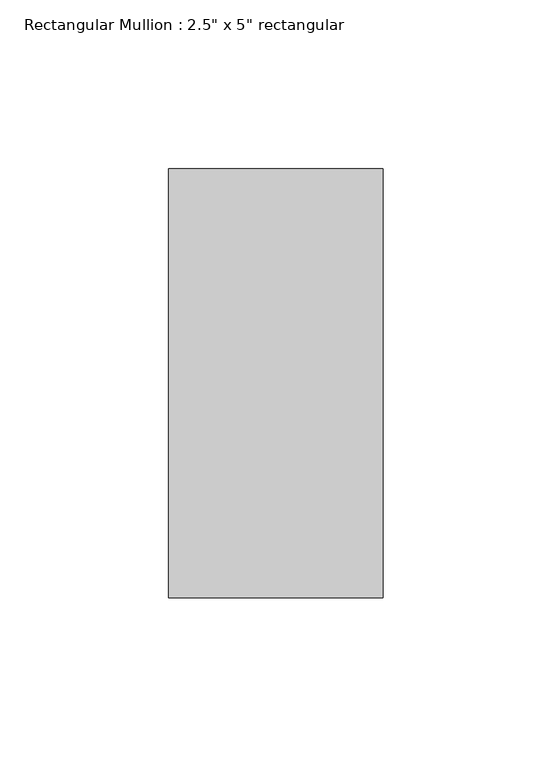
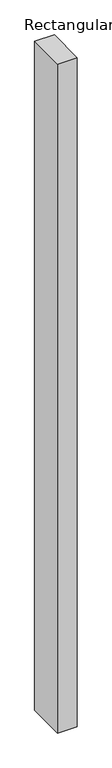
"""IFC4 building model written with IfcOpenShell, lengths in millimetres: member geometry."""

from ifc_helpers import new_model, si_unit, frame, origin, place, context, project, spatial, polyline, outline, extrude, source, transform, mapped, element, save


def member_cc169a76(model_context):
    return source(origin(), model_context, "Body", "SweptSolid", [
        extrude(outline(polyline([(0.0, 63.5), (0.0, -63.5), (-63.5, -63.5), (-63.5, 63.5), (0.0, 63.5)])), frame((0.0, 0.0, -2279.5655837), z_axis=(0.0, 0.0, 1.0), x_axis=(1.0, 0.0, 0.0)), (0.0, 0.0, 1.0), 2279.5655837),
    ])


if __name__ == "__main__":
    model = new_model("IFC4")
    model_context = context("Model", 3, world=origin())
    ifc_project = project(units=[si_unit("LENGTHUNIT", "METRE", prefix="MILLI")], contexts=[model_context])
    site = spatial("IfcSite", under=ifc_project)
    building = spatial("IfcBuilding", under=site)
    placement = place(None, origin())
    member_shape = member_cc169a76(model_context)
    element("IfcMember", 1, ObjectType="Rectangular Mullion : 2.5\" x 5\" rectangular", at=placement, inside=building, context=model_context, shape_type="MappedRepresentation", body=[
        mapped(member_shape, transform((0.0, 0.0, 0.0), x_axis=(1.0, 0.0, 0.0), y_axis=(0.0, 1.0, 0.0), z_axis=(0.0, 0.0, 1.0))),
    ])
    save(model, "model.ifc")

# Revit data of these elements
# Type "Rectangular Mullion : 2.5\" x 5\" rectangular"
#   built-in parameter 1007304 = 0.416667 (stored number, unit not read)
#   built-in parameter 1007301 = 0.104167 (stored number, unit not read)
#   built-in parameter 1007300 = 0.104167 (stored number, unit not read)
# Element 1 (IfcMember, "Rectangular Mullion : 2.5\" x 5\" rectangular")
#   Materials on its faces: "Aluminum"
# Materials
#   "Aluminum": class "Metal", colour RGB 247 247 247, transparency 0, Description = "Aluminum 6061", Cost = 0
